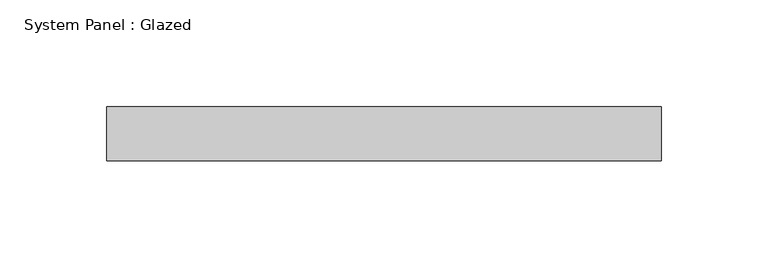
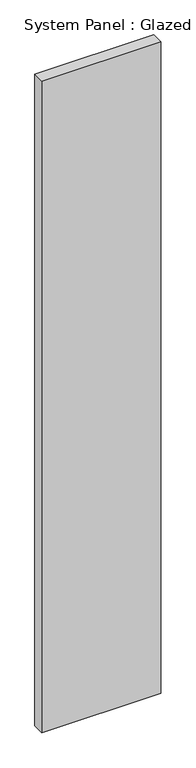
"""IFC4 building model written with IfcOpenShell, lengths in millimetres: plate geometry, System Panel : Glazed."""

from ifc_helpers import new_model, si_unit, origin, origin_with_axes, place, context, project, spatial, polyline, outline, extrude, source, transform, mapped, element, save


def system_panel_glazed_012e7337(model_context):
    return source(origin(), model_context, "Body", "SweptSolid", [
        extrude(outline(polyline([(130.175, 19.05), (-130.175, 19.05), (-130.175, 44.45), (130.175, 44.45), (130.175, 19.05)])), origin_with_axes(), (0.0, 0.0, 1.0), 1507.3549218),
    ])


if __name__ == "__main__":
    model = new_model("IFC4")
    model_context = context("Model", 3, world=origin())
    ifc_project = project(units=[si_unit("LENGTHUNIT", "METRE", prefix="MILLI")], contexts=[model_context])
    site = spatial("IfcSite", under=ifc_project)
    building = spatial("IfcBuilding", under=site)
    placement = place(None, origin())
    system_panel_glazed_shape = system_panel_glazed_012e7337(model_context)
    element("IfcPlate", 1, ObjectType="System Panel : Glazed", at=placement, inside=building, context=model_context, shape_type="MappedRepresentation", body=[
        mapped(system_panel_glazed_shape, transform((0.0, 0.0, 0.0), x_axis=(1.0, 0.0, 0.0), y_axis=(0.0, 1.0, 0.0), z_axis=(0.0, 0.0, 1.0))),
    ])
    save(model, "model.ifc")

# Revit data of these elements
# Type "System Panel : Glazed"
#   Construction Type Id = "GSP4R"
#   Analytic Construction = "1/8 in Pilkington single glazing"
#   Visual Light Transmittance = 0.9
#   Solar Heat Gain Coefficient = 0.86
#   Heat Transfer Coefficient (U) = 1.18115 BTU/(h·ft²·°F)
#   Define Thermal Properties by = 1
# Element 1 (IfcPlate, "System Panel : Glazed")
#   Materials on its faces: "Glass"
# Materials
#   "Glass": class "Glass", colour RGB 0 128 192, transparency 0.75, Description = "Soda Lime Glass", Cost = 0
